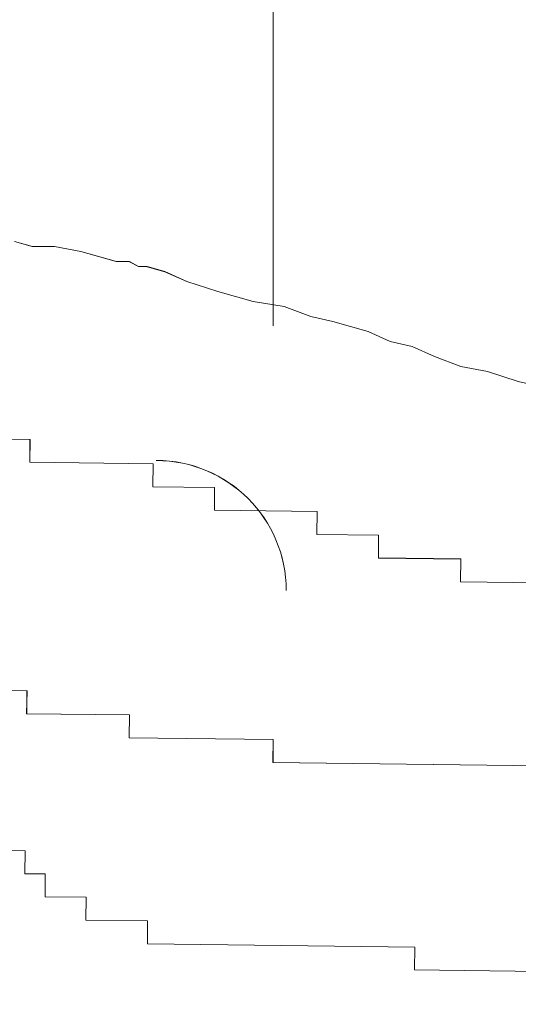
# Model space of a CAD drawing. Units: inches. Extents: x -466983 to 1020, y 324 to 318697.
# Tile 61 of 97: x 634.801 to 637.815, y 942.694 to 948.644. Entities that reach past the tile are written whole.
import ezdxf

# ---------------------------------------------------------------- set-up
doc = ezdxf.new("R2010")
doc.units = ezdxf.units.IN
doc.header["$MEASUREMENT"] = 0
doc.layers.add('A-FLOR-PATT', color=252, linetype='Continuous', lineweight=13)
doc.layers.add('A-FURN', color=8, linetype='Continuous', lineweight=18)

# ---------------------------------------------------------------- blocks, each defined once
blk = doc.blocks.new('L Shaped Sofa')
at = {"ltscale": 2}
for p, q in [((2423.757, 743.446), (2430.788, 743.36)), ((2430.788, 743.36), (2430.785, 743.108)), ((2430.785, 743.108), (2433.734, 743.072)), ((2433.734, 743.072), (2433.731, 742.82)), ((2433.731, 742.82), (2434.412, 742.812)), ((2434.412, 742.812), (2434.409, 742.56)), ((2434.409, 742.56), (2434.862, 742.555)), ((2434.862, 742.555), (2434.859, 742.303)), ((2434.859, 742.303), (2435.086, 742.3)), ((2435.086, 742.3), (2435.083, 742.048)), ((2435.083, 742.048), (2435.764, 742.04)), ((2421.46, 741.207), (2432.349, 741.074)), ((2432.349, 741.074), (2432.346, 740.822)), ((2432.346, 740.822), (2433.933, 740.802)), ((2433.933, 740.802), (2433.93, 740.55)), ((2433.93, 740.55), (2435.065, 740.536)), ((2435.065, 740.536), (2435.061, 740.285)), ((2435.061, 740.285), (2435.515, 740.279)), ((2428.468, 739.105), (2430.282, 739.083)), ((2430.282, 739.083), (2430.279, 738.831)), ((2430.279, 738.831), (2431.187, 738.82)), ((2431.187, 738.82), (2431.184, 738.568)), ((2431.184, 738.568), (2431.864, 738.56)), ((2431.864, 738.56), (2431.861, 738.308)), ((2431.861, 738.308), (2432.995, 738.294)), ((2432.995, 738.294), (2432.992, 738.042)), ((2432.992, 738.042), (2433.673, 738.034)), ((2433.673, 738.034), (2433.67, 737.782)), ((2433.67, 737.782), (2435.031, 737.765)), ((2435.031, 737.765), (2435.028, 737.514)), ((2435.028, 737.514), (2436.389, 737.497)), ((2429.4, 736.93), (2429.644, 736.875)), ((2429.644, 736.875), (2429.985, 736.765)), ((2429.985, 736.765), (2430.277, 736.709)), ((2430.277, 736.709), (2430.569, 736.599)), ((2430.569, 736.599), (2430.813, 736.49)), ((2430.813, 736.49), (2431.056, 736.434)), ((2431.056, 736.434), (2431.3, 736.325)), ((2431.3, 736.325), (2431.689, 736.215)), ((2431.689, 736.215), (2431.933, 736.159)), ((2432.347, 728.35), (2432.347, 736.259)), ((2431.933, 736.159), (2432.225, 736.049)), ((2432.225, 736.049), (2432.566, 735.994)), ((2432.566, 735.994), (2432.956, 735.883)), ((2432.956, 735.883), (2433.297, 735.773)), ((2433.297, 735.773), (2433.54, 735.664)), ((2433.54, 735.664), (2433.735, 735.609)), ((2433.735, 735.609), (2433.833, 735.608)), ((2433.833, 735.608), (2433.93, 735.554)), ((2433.93, 735.554), (2434.076, 735.553)), ((2434.076, 735.553), (2434.466, 735.443)), ((2434.466, 735.443), (2434.758, 735.387)), ((2434.758, 735.387), (2435.002, 735.386)), ((2435.002, 735.386), (2435.197, 735.331))]:
    blk.add_line(p, q, dxfattribs=at)
blk.add_arc((2433.636, 739.178), 1.433, 180, 270, dxfattribs=at)

msp = doc.modelspace()

# ---------------------------------------------------------------- hatches: boundary and pattern name
at = {"layer": 'A-FLOR-PATT', "transparency": 33554572}
h = msp.add_hatch(dxfattribs=at)
h.set_pattern_fill('ANSI37', color=256, scale=30)
h.set_pattern_definition([(45, (-1212.4137, -290.035), (-2.6516504, 2.6516504), []), (135, (-1212.4137, -290.035), (-2.6516504, -2.6516504), [])])
h.paths.add_polyline_path([(901.8057, 1075.9377), (900.6144, 1075.9377), (900.6144, 1065.3856), (899.391, 1065.3856), (898.0911, 1065.3856), (892.8356, 1058.7098, -0.258377), (892.1875, 1058.3509), (879.9848, 1058.3509, -0.20177), (879.4382, 1058.5808), (874.0812, 1065.3856), (872.7813, 1065.3856), (871.5579, 1065.3856), (871.5579, 1075.9377), (813.8057, 1075.9377), (813.8057, 1044.7922), (832.3947, 1044.7922, -0.394795), (848.6602, 1028.5356), (848.6602, 1009.9377), (901.8057, 1009.9377), (901.8057, 1015.9377), (901.3057, 1015.9377), (871.3057, 1015.9377), (871.3057, 1017.2502), (871.3344, 1017.2502, -0.401453), (901.3057, 1045.9377), (901.8057, 1045.9377)])
edge = h.paths.add_edge_path(flags=16)
edge.add_line((847.7731, 1068.9486), (847.7731, 1073.7088))
edge.add_arc((849.2269, 1073.7088), 1.4538, 90, 180, ccw=False)
edge.add_line((849.2269, 1075.1627), (864.4921, 1075.1627))
edge.add_arc((864.4921, 1073.7088), 1.4538, 0, 90, ccw=False)
edge.add_line((865.9459, 1073.7088), (865.9459, 1069.0035))
edge.add_arc((832.6447, 1068.9761), 33.3012, -20.61234, 0.04725, ccw=False)
edge.add_ellipse((856.8595, 1058.48), major_axis=(0, 10.2131), ratio=0.6859192, start_angle=100.00884, end_angle=259.99116, ccw=False)
edge.add_arc((881.0742, 1068.9761), 33.3012, 180.04725, 200.61234, ccw=False)
h.paths.add_polyline_path([(853.1456, 1066.4815), (853.1456, 1066.4534), (853.1463, 1066.4534, 0.433107), (852.9166, 1066.6849), (852.9166, 1066.4534), (853.1456, 1066.4534), (853.1456, 1066.4815), (853.088, 1066.6122, 0.697939), (852.6995, 1066.4534), (852.7003, 1066.4534), (852.7003, 1066.4815), (852.9166, 1067.0012), (852.9166, 1066.6849, -0.396254)], flags=0)
h.paths.add_polyline_path([(861.0187, 1066.4815), (861.0187, 1066.4534), (861.0194, 1066.4534, 0.416404), (860.8024, 1066.6849), (860.8024, 1066.4534), (861.0187, 1066.4534), (861.0187, 1066.4815), (860.9672, 1066.6053, 0.713344), (860.5726, 1066.4534), (860.5734, 1066.4534), (860.5734, 1066.4815), (860.8024, 1067.0012), (860.8024, 1066.6849, -0.379973)], flags=0)
edge = h.paths.add_edge_path(flags=0)
edge.add_spline(control_points=[(861.1298, 1065.7855), (861.4661, 1065.2478), (861.6134, 1065.0161), (861.9833, 1064.3736), (862.1924, 1063.9443), (862.5614, 1063.0391), (862.7212, 1062.5633), (862.9865, 1061.5781), (863.092, 1061.0689), (863.2452, 1060.031), (863.293, 1059.5025), (863.3295, 1058.4409), (863.3181, 1057.9078), (863.2366, 1056.8518), (863.1664, 1056.3289), (862.9695, 1055.308), (862.8427, 1054.8099), (862.5365, 1053.8522), (862.3571, 1053.3927), (861.9514, 1052.5249), (861.7251, 1052.1166), (861.233, 1051.3622), (860.9672, 1051.0162), (860.4048, 1050.3949), (860.1082, 1050.1197), (859.4937, 1049.6461), (859.1758, 1049.4476), (858.5276, 1049.1299), (858.1973, 1049.0107), (857.5315, 1048.8518), (857.1959, 1048.8121), (856.5249, 1048.812), (856.1894, 1048.8515), (855.5236, 1049.0101), (855.1933, 1049.1291), (854.545, 1049.4465), (854.2271, 1049.6449), (853.6124, 1050.1183), (853.3158, 1050.3933), (852.7533, 1051.0143), (852.4874, 1051.3602), (851.9952, 1052.1144), (851.7688, 1052.5225), (851.3629, 1053.3902), (851.1834, 1053.8496), (850.877, 1054.8071), (850.7501, 1055.3051), (850.553, 1056.326), (850.4827, 1056.8488), (850.401, 1057.9048), (850.3895, 1058.4379), (850.4257, 1059.4995), (850.4734, 1060.0281), (850.6265, 1061.066), (850.7318, 1061.5753), (850.9969, 1062.5605), (851.1567, 1063.0365), (851.5254, 1063.9418), (851.7345, 1064.3712), (852.1056, 1065.0164), (852.2544, 1065.2503), (852.6082, 1065.7335)], knot_values=[3.915332, 3.915332, 3.915332, 3.915332, 4.013468, 4.013468, 4.175532, 4.175532, 4.337596, 4.337596, 4.49966, 4.49966, 4.661724, 4.661724, 4.823788, 4.823788, 4.985852, 4.985852, 5.147916, 5.147916, 5.30998, 5.30998, 5.472044, 5.472044, 5.634109, 5.634109, 5.796173, 5.796173, 5.958237, 5.958237, 6.120301, 6.120301, 6.282365, 6.282365, 6.444429, 6.444429, 6.606493, 6.606493, 6.768557, 6.768557, 6.930621, 6.930621, 7.092685, 7.092685, 7.254749, 7.254749, 7.416813, 7.416813, 7.578878, 7.578878, 7.740942, 7.740942, 7.903006, 7.903006, 8.06507, 8.06507, 8.227134, 8.227134, 8.389198, 8.389198, 8.551262, 8.551262, 8.65037, 8.65037, 8.65037, 8.65037], degree=3, periodic=0)
edge.add_line((852.6421, 1065.7855), (861.1298, 1065.7855))
edge = h.paths.add_edge_path(flags=0)
edge.add_ellipse((856.8496, 1057.7432), major_axis=(0, 7.7921), ratio=0.687861, start_angle=0, end_angle=360)
h.paths.add_polyline_path([(848.8634, 1069.3891), (848.8634, 1073.9605, -0.414214), (849.9538, 1075.0508), (863.7652, 1075.0508, -0.414214), (864.8555, 1073.9605), (864.8555, 1069.3891, -0.388936), (864.5237, 1069.027, -0.043561), (849.1953, 1069.027, -0.388936)], flags=0)
h.paths.add_polyline_path([(853.1006, 1068.1122, -1), (852.6775, 1068.1122, -1)], flags=0)
edge = h.paths.add_edge_path(flags=0)
edge.add_ellipse((856.8595, 1057.3378), major_axis=(0, 2.207), ratio=0.657164, start_angle=0, end_angle=360)
h.paths.add_polyline_path([(861.0415, 1068.1122, -1), (860.6184, 1068.1122, -1)], flags=0)
edge = h.paths.add_edge_path()
edge.add_line((573.9537, 1057.3412), (573.9537, 1075.9377))
edge.add_line((573.9537, 1075.9377), (558.7308, 1075.9377))
edge.add_line((558.7308, 1075.9377), (558.7308, 1065.3856))
edge.add_line((558.7308, 1065.3856), (557.5074, 1065.3856))
edge.add_line((557.5074, 1065.3856), (556.2075, 1065.3856))
edge.add_line((556.2075, 1065.3856), (550.952, 1058.7098))
edge.add_arc((550.3039, 1059.1155), 0.7646, 270, 327.94832, ccw=False)
edge.add_line((550.3039, 1058.3509), (538.1012, 1058.3509))
edge.add_arc((538.1012, 1059.1155), 0.7646, 224.3704, 270, ccw=False)
edge.add_line((537.5546, 1058.5808), (532.1976, 1065.3856))
edge.add_line((532.1976, 1065.3856), (530.8977, 1065.3856))
edge.add_line((530.8977, 1065.3856), (529.6743, 1065.3856))
edge.add_line((529.6743, 1065.3856), (529.6743, 1075.9377))
edge.add_line((529.6743, 1075.9377), (520.8057, 1075.9377))
edge.add_line((520.8057, 1075.9377), (520.8057, 1045.9377))
edge.add_line((520.8057, 1045.9377), (521.3057, 1045.9377))
edge.add_arc((521.3057, 1015.9377), 30, 2.50749, 90, ccw=False)
edge.add_line((551.277, 1017.2502), (551.3057, 1017.2502))
edge.add_line((551.3057, 1017.2502), (551.3057, 1015.9377))
edge.add_line((551.3057, 1015.9377), (520.8057, 1015.9377))
edge.add_line((520.8057, 1015.9377), (520.8057, 1009.9377))
edge.add_line((520.8057, 1009.9377), (559.1913, 1010.4022))
edge.add_arc((559.1913, 1011.856), 1.4538, 180, 270, ccw=False)
edge.add_line((557.7375, 1011.856), (557.7375, 1016.5613))
edge.add_arc((591.0386, 1016.5888), 33.3012, 159.38766, 180.04725, ccw=False)
edge.add_ellipse((566.8239, 1027.0848), major_axis=(0, 10.2131), ratio=0.6859192, start_angle=280.00884, end_angle=439.99116, ccw=False)
edge.add_arc((542.6091, 1016.5888), 33.3012, 0.04725, 20.61234, ccw=False)
edge.add_line((575.9103, 1016.6162), (575.9103, 1011.856))
edge.add_arc((574.4565, 1011.856), 1.4538, -90, 0, ccw=False)
edge.add_line((574.4565, 1010.4022), (608.8057, 1009.9377))
edge.add_line((608.8057, 1009.9377), (608.8057, 1041.0857))
edge.add_line((608.8057, 1041.0857), (590.2179, 1041.0857))
edge.add_arc((590.775, 1057.9074), 16.8309, 181.92775, 268.10321, ccw=False)
edge = h.paths.add_edge_path()
edge.add_ellipse((494.2443, 583.6204), major_axis=(0, 10.2131), ratio=0.6859192, start_angle=280.00884, end_angle=439.99116, ccw=False)
edge.add_arc((470.0296, 573.1243), 33.3012, 0.04725, 20.61234, ccw=False)
edge.add_line((503.3307, 573.1518), (503.3307, 568.3916))
edge.add_arc((501.8769, 568.3916), 1.4538, -90, 0, ccw=False)
edge.add_line((501.8769, 566.9377), (539.8057, 566.9377))
edge.add_line((539.8057, 566.9377), (539.8057, 572.9377))
edge.add_line((539.8057, 572.9377), (539.3057, 572.9377))
edge.add_line((539.3057, 572.9377), (509.3057, 572.9377))
edge.add_line((509.3057, 572.9377), (509.3057, 574.2502))
edge.add_line((509.3057, 574.2502), (509.3344, 574.2502))
edge.add_arc((539.3057, 572.9377), 30, 90, 177.49251, ccw=False)
edge.add_line((539.3057, 602.9377), (539.8057, 602.9377))
edge.add_line((539.8057, 602.9377), (539.8057, 626.9377))
edge.add_line((539.8057, 626.9377), (531.7718, 626.9377))
edge.add_line((531.7718, 626.9377), (531.7718, 616.3856))
edge.add_line((531.7718, 616.3856), (530.5484, 616.3856))
edge.add_line((530.5484, 616.3856), (529.2485, 616.3856))
edge.add_line((529.2485, 616.3856), (523.7105, 609.3509))
edge.add_line((523.7105, 609.3509), (510.7766, 609.3509))
edge.add_line((510.7766, 609.3509), (505.2386, 616.3856))
edge.add_line((505.2386, 616.3856), (503.9387, 616.3856))
edge.add_line((503.9387, 616.3856), (502.7153, 616.3856))
edge.add_line((502.7153, 616.3856), (502.7153, 626.9377))
edge.add_line((502.7153, 626.9377), (481.6983, 626.9377))
edge.add_line((481.6983, 626.9377), (481.6983, 610.995))
edge.add_arc((467.2703, 611.4728), 14.4359, 271.92775, 358.10321, ccw=False)
edge.add_line((467.7559, 597.0451), (451.8057, 597.0451))
edge.add_line((451.8057, 597.0451), (451.8057, 584.4035))
edge.add_line((451.8057, 584.4035), (451.8057, 566.9377))
edge.add_line((451.8057, 566.9377), (486.6117, 566.9377))
edge.add_arc((486.6117, 568.3916), 1.4538, 180, 270, ccw=False)
edge.add_line((485.1579, 568.3916), (485.1579, 573.0969))
edge.add_arc((518.4591, 573.1243), 33.3012, 159.38766, 180.04725, ccw=False)
h.paths.add_polyline_path([(836.2609, 1020.7328), (879.8898, 1020.7328), (879.8898, 1039.3902), (836.2609, 1039.3902)], flags=25)
h.paths.add_polyline_path([(549.9851, 1036.7492), (593.614, 1036.7492), (593.614, 1055.4065), (549.9851, 1055.4065)], flags=24)
h.paths.add_polyline_path([(475.123, 595.5959), (518.752, 595.5959), (518.752, 614.2532), (475.123, 614.2532)], flags=24)
h = msp.add_hatch(dxfattribs=at)
h.set_pattern_fill('ANSI37', color=256, scale=20)
h.set_pattern_definition([(45, (-1212.4137, -290.035), (-1.767767, 1.767767), []), (135, (-1212.4137, -290.035), (-1.767767, -1.767767), [])])
h.paths.add_polyline_path([(809.8057, 870.9377), (809.8057, 888.1519), (806.9985, 888.1519), (802.6624, 888.1519), (789.3832, 888.1519), (786.2846, 888.1519, -0.414214), (785.4991, 888.9374), (785.4991, 900.1959), (785.4991, 908.4696, -0.414214), (786.8082, 909.7787, -0.414214), (785.4991, 911.0878), (785.4991, 929.1015, -0.414214), (786.8082, 930.4106, -0.414214), (785.4991, 931.7197), (785.4991, 931.9039, -0.414214), (784.19, 930.5948), (766.7223, 930.5948, -0.412359), (765.4132, 931.8956, -0.413741), (764.1145, 930.5782), (744.5781, 930.422, -0.416556), (743.7864, 931.2075), (743.7864, 933.5153), (742.2154, 933.5153), (742.2154, 952.024, -0.001344), (743.7864, 952.1998), (743.7864, 953.9377), (678.5915, 953.9377), (678.5915, 951.1305), (678.5915, 946.7945), (678.5915, 933.5153), (678.5915, 930.4166, -0.414214), (677.806, 929.6312), (666.5475, 929.6312), (658.2738, 929.6312, -0.414214), (656.9647, 930.9403, -0.414214), (655.6556, 929.6312), (637.6419, 929.6312, -0.414214), (636.3328, 930.9403, -0.414214), (635.0237, 929.6312), (634.8395, 929.6312, -0.414214), (636.1486, 928.322), (636.1486, 910.8544, -0.412359), (634.8478, 909.5452, -0.413741), (636.1653, 908.2466), (636.3214, 888.7102, -0.416556), (635.5359, 887.9184), (633.2281, 887.9184), (633.2281, 886.3475), (614.7194, 886.3475, -0.001344), (614.5436, 887.9184), (612.8057, 887.9184), (612.8057, 834.9377), (612.8057, 752.9377), (612.8057, 748.9377), (612.8057, 697.9377), (654.8057, 697.9377), (654.8057, 701.9377), (715.8057, 701.9377), (715.8057, 737.4353), (774.2918, 737.4353), (774.2918, 795.9377), (809.8057, 795.9377)])
h.paths.add_polyline_path([(679.2761, 849.5757, 0.102523), (682.1475, 849.2608, -0.080461), (694.5428, 849.7725, -0.283899), (694.4822, 849.0082, 0.136605), (694.4068, 848.8103, -0.030441), (694.5428, 846.8929), (694.5428, 842.6198), (694.5428, 838.3466, -0.028219), (694.4246, 836.5684), (694.425, 836.5684, 0.196187), (694.4456, 836.2708, -0.302897), (694.5428, 835.467, -0.080461), (682.1475, 835.9787, 0.102523), (679.2761, 835.6638, -0.58611), (678.6457, 836.0169), (678.6457, 849.2227, -0.58611)], flags=16)
h.paths.add_polyline_path([(679.5173, 848.6515, 0.699597), (679.476, 848.6342, 1.20716), (679.1935, 848.7422, 0.010621)], flags=0)
h.paths.add_polyline_path([(679.4923, 836.5608, -0.013798), (679.9178, 836.6594, -0.071703), (682.8533, 837.1434, -0.165743), (682.1665, 839.1006), (682.1665, 842.6094), (682.1665, 846.0603, -0.240616), (683.4733, 848.6767, -0.068263), (693.9295, 849.0082), (693.7875, 848.7083), (693.7875, 849.0228, 0.067332), (683.4733, 848.6767, 0.240616), (682.1665, 846.0603), (682.1665, 842.6094), (682.1665, 839.1006, 0.23459), (683.461, 836.5513, 0.068093), (693.7875, 836.1955), (693.7875, 836.5104), (693.9296, 836.2102, -0.077215), (682.2421, 836.7815, 0.086627), (679.5283, 836.5701, -0.628402), (679.5029, 836.5735), (679.5029, 836.6071, 0.910458)], flags=0)
h.paths.add_polyline_path([(679.476, 848.6364), (679.2069, 848.647), (679.2069, 836.5718, 0.913566), (679.3645, 836.5861), (679.476, 836.5824)], flags=0)
h.paths.add_polyline_path([(679.2761, 829.8604, 0.102523), (682.1475, 829.5455, -0.080461), (694.5428, 830.0572, -0.283899), (694.4822, 829.2929, 0.136605), (694.4068, 829.095, -0.030441), (694.5428, 827.1776), (694.5428, 822.9045), (694.5428, 818.6314, -0.028219), (694.4246, 816.8531), (694.425, 816.8532, 0.196187), (694.4456, 816.5555, -0.302897), (694.5428, 815.7517, -0.080461), (682.1475, 816.2635, 0.102523), (679.2761, 815.9485, -0.58611), (678.6457, 816.3016), (678.6457, 829.5074, -0.58611)], flags=16)
h.paths.add_polyline_path([(679.5173, 828.9362, 0.699597), (679.476, 828.9189, 1.20716), (679.1935, 829.0269, 0.010621)], flags=0)
h.paths.add_polyline_path([(679.4923, 816.8456, -0.013798), (679.9178, 816.9441, -0.071703), (682.8533, 817.4281, -0.165743), (682.1665, 819.3853), (682.1665, 822.8941), (682.1665, 826.345, -0.240616), (683.4733, 828.9614, -0.068263), (693.9295, 829.2929), (693.7875, 828.9931), (693.7875, 829.3076, 0.067332), (683.4733, 828.9614, 0.240616), (682.1665, 826.345), (682.1665, 822.8941), (682.1665, 819.3853, 0.23459), (683.461, 816.836, 0.068093), (693.7875, 816.4802), (693.7875, 816.7952), (693.9296, 816.4949, -0.077215), (682.2421, 817.0662, 0.086627), (679.5283, 816.8549, -0.628402), (679.5029, 816.8582), (679.5029, 816.8918, 0.910458)], flags=0)
h.paths.add_polyline_path([(679.476, 828.9211), (679.2069, 828.9317), (679.2069, 816.8565, 0.913566), (679.3645, 816.8708), (679.476, 816.8671)], flags=0)
h.paths.add_polyline_path([(679.2761, 810.1451, 0.102523), (682.1475, 809.8302, -0.080461), (694.5428, 810.342, -0.3023), (694.4466, 809.5394, 0.10023), (694.4058, 809.3878, -0.03057), (694.5428, 807.4623), (694.5428, 803.1892), (694.5428, 798.9161, -0.03057), (694.4058, 796.9906, 0.10023), (694.4466, 796.839, -0.3023), (694.5428, 796.0365, -0.080461), (682.1475, 796.5482, 0.102523), (679.2761, 796.2333, -0.58611), (678.6457, 796.5863), (678.6457, 809.7921, -0.58611)], flags=16)
h.paths.add_polyline_path([(679.5173, 809.2417, 0.699597), (679.476, 809.2244, 1.20716), (679.1935, 809.3324, 0.010621)], flags=0)
h.paths.add_polyline_path([(679.4923, 797.151, -0.013798), (679.9178, 797.2496, -0.071703), (682.8533, 797.7336, -0.165743), (682.1665, 799.6908), (682.1665, 803.1996), (682.1665, 806.6505, -0.239349), (683.461, 809.2577, -0.072465), (694.4468, 809.5405, 0.197932), (694.425, 809.2405), (693.7875, 809.2985), (693.7875, 809.6135, 0.068093), (683.461, 809.2577, 0.239349), (682.1665, 806.6505), (682.1665, 803.1996), (682.1665, 799.6908, 0.235854), (683.4733, 797.1323, 0.067332), (693.7875, 796.7861), (693.7875, 797.1006), (694.425, 797.1586, 0.197932), (694.4468, 796.8586, -0.080419), (682.1557, 797.3795, 0.083867), (679.5283, 797.1603, -0.628402), (679.5029, 797.1637), (679.5029, 797.1973, 0.910458)], flags=0)
h.paths.add_polyline_path([(679.2069, 809.2372), (679.2069, 797.162, 0.913566), (679.3645, 797.1763), (679.476, 797.1726), (679.476, 809.2266)], flags=0)
h.paths.add_polyline_path([(695.3643, 853.2989), (728.2231, 853.2989), (728.2231, 771.1519), (695.3643, 771.1519)], flags=16)
h.paths.add_polyline_path([(696.0215, 852.6417), (727.5659, 852.6417), (727.5659, 771.809), (696.0215, 771.809)], flags=0)
h.paths.add_polyline_path([(679.2761, 788.7869, 0.102523), (682.1475, 788.472, -0.080461), (694.5428, 788.9837, -0.3023), (694.4466, 788.1812, 0.10023), (694.4058, 788.0296, -0.03057), (694.5428, 786.1041), (694.5428, 781.831), (694.5428, 777.5578, -0.03057), (694.4058, 775.6323, 0.10023), (694.4466, 775.4808, -0.3023), (694.5428, 774.6782, -0.080461), (682.1475, 775.19, 0.102523), (679.2761, 774.875, -0.58611), (678.6457, 775.2281), (678.6457, 788.4339, -0.58611)], flags=16)
h.paths.add_polyline_path([(679.5173, 787.8834, 0.699597), (679.476, 787.8662, 1.20716), (679.1935, 787.9742, 0.010621)], flags=0)
h.paths.add_polyline_path([(679.4923, 775.7928, -0.013798), (679.9178, 775.8914, -0.071703), (682.8533, 776.3753, -0.165743), (682.1665, 778.3325), (682.1665, 781.8414), (682.1665, 785.2922, -0.239349), (683.461, 787.8995, -0.072465), (694.4468, 788.1823, 0.197932), (694.425, 787.8823), (693.7875, 787.9403), (693.7875, 788.2553, 0.068093), (683.461, 787.8995, 0.239349), (682.1665, 785.2922), (682.1665, 781.8414), (682.1665, 778.3325, 0.235854), (683.4733, 775.7741, 0.067332), (693.7875, 775.4279), (693.7875, 775.7424), (694.425, 775.8004, 0.197932), (694.4468, 775.5004, -0.080419), (682.1557, 776.0212, 0.083867), (679.5283, 775.8021, -0.628402), (679.5029, 775.8054), (679.5029, 775.8391, 0.910458)], flags=0)
h.paths.add_polyline_path([(679.2069, 787.8789), (679.2069, 775.8038, 0.913566), (679.3645, 775.818), (679.476, 775.8144), (679.476, 787.8684)], flags=0)
h.paths.add_polyline_path([(704.641, 854.1204, -0.080461), (705.1527, 866.5157, 0.102523), (704.8378, 869.3871, -0.58611), (705.1908, 870.0174), (718.3966, 870.0174, -0.58611), (718.7496, 869.3871, 0.102523), (718.4347, 866.5157, -0.080461), (718.9465, 854.1204, -0.3023), (718.1439, 854.2166, 0.10023), (717.9924, 854.2574, -0.03057), (716.0668, 854.1204), (711.7937, 854.1204), (707.5206, 854.1204, -0.03057), (705.5951, 854.2574, 0.10023), (705.4435, 854.2166, -0.3023)], flags=16)
h.paths.add_polyline_path([(717.8462, 869.1459, 0.699597), (717.8289, 869.1872, 1.20716), (717.9369, 869.4697, 0.010621)], flags=0)
h.paths.add_polyline_path([(705.4631, 854.2164, -0.080419), (705.984, 866.5074, 0.083867), (705.7648, 869.1349, -0.628402), (705.7682, 869.1603), (705.8018, 869.1603, 0.910458), (705.7555, 869.1709, -0.013798), (705.8541, 868.7454, -0.071703), (706.3381, 865.8099, -0.165743), (708.2953, 866.4967), (711.8041, 866.4967), (715.255, 866.4967, -0.239349), (717.8622, 865.2022, -0.072465), (718.145, 854.2164, 0.197932), (717.845, 854.2382), (717.903, 854.8757), (718.218, 854.8757, 0.068093), (717.8622, 865.2022, 0.239349), (715.255, 866.4967), (711.8041, 866.4967), (708.2953, 866.4967, 0.235854), (705.7368, 865.1898, 0.067332), (705.3906, 854.8757), (705.7051, 854.8757), (705.7631, 854.2382, 0.197932)], flags=16)
h.paths.add_polyline_path([(705.7665, 869.4563, 0.913566), (705.7808, 869.2987), (705.7771, 869.1872), (717.8311, 869.1872), (717.8417, 869.4563)], flags=0)
h.paths.add_polyline_path([(729.0446, 842.6198), (729.0446, 846.8929, -0.03057), (729.1817, 848.8184, 0.10023), (729.1408, 848.9699, -0.3023), (729.0446, 849.7725, -0.080461), (741.4399, 849.2608, 0.102523), (744.3113, 849.5757, -0.58611), (744.9417, 849.2227), (744.9417, 836.0169, -0.58611), (744.3113, 835.6638, 0.102523), (741.4399, 835.9787, -0.080461), (729.0446, 835.467, -0.3023), (729.1408, 836.2696, 0.10023), (729.1817, 836.4211, -0.03057), (729.0446, 838.3466)], flags=16)
h.paths.add_polyline_path([(744.1115, 836.5846, 1.20716), (744.3939, 836.4766, 0.010621), (744.0701, 836.5673, 0.699597)], flags=0)
h.paths.add_polyline_path([(729.1407, 836.2684, 0.197932), (729.1624, 836.5684), (729.7999, 836.5104), (729.7999, 836.1955, 0.068093), (740.1264, 836.5513, 0.239349), (741.4209, 839.1585), (741.4209, 842.6094), (741.4209, 846.1182, 0.235854), (740.1141, 848.6767, 0.067332), (729.7999, 849.0228), (729.7999, 848.7083), (729.1624, 848.6503, 0.197932), (729.1407, 848.9504, -0.080419), (741.4317, 848.4295, 0.083867), (744.0591, 848.6486, -0.628402), (744.0845, 848.6453), (744.0845, 848.6117, 0.910458), (744.0951, 848.6579, -0.013798), (743.6696, 848.5594, -0.071703), (740.7341, 848.0754, -0.165743), (741.4209, 846.1182), (741.4209, 842.6094), (741.4209, 839.1585, -0.239349), (740.1264, 836.5513, -0.072465)], flags=0)
h.paths.add_polyline_path([(729.0446, 830.0572, -0.080461), (741.4399, 829.5455, 0.102523), (744.3113, 829.8604, -0.58611), (744.9417, 829.5074), (744.9417, 816.3016, -0.58611), (744.3113, 815.9485, 0.102523), (741.4399, 816.2635, -0.080461), (729.0446, 815.7517, -0.3023), (729.1408, 816.5543, 0.10023), (729.1817, 816.7058, -0.03057), (729.0446, 818.6314), (729.0446, 822.9045), (729.0446, 827.1776, -0.03057), (729.1817, 829.1031, 0.10023), (729.1408, 829.2547, -0.3023)], flags=16)
h.paths.add_polyline_path([(744.1115, 816.8693, 1.20716), (744.3939, 816.7613, 0.010621), (744.0701, 816.852, 0.699597)], flags=0)
h.paths.add_polyline_path([(729.1407, 829.2351, -0.080419), (741.4317, 828.7142, 0.083867), (744.0591, 828.9334, -0.628402), (744.0845, 828.93), (744.0845, 828.8964, 0.910458), (744.0951, 828.9427, -0.013798), (743.6696, 828.8441, -0.071703), (740.7341, 828.3601, -0.165743), (741.4209, 826.4029), (741.4209, 822.8941), (741.4209, 819.4432, -0.239349), (740.1264, 816.836, -0.072465), (729.1407, 816.5531, 0.197932), (729.1624, 816.8532), (729.7999, 816.7952), (729.7999, 816.4802, 0.068093), (740.1264, 816.836, 0.239349), (741.4209, 819.4432), (741.4209, 822.8941), (741.4209, 826.4029, 0.235854), (740.1141, 828.9614, 0.067332), (729.7999, 829.3076), (729.7999, 828.9931), (729.1624, 828.9351, 0.197932)], flags=16)
h.paths.add_polyline_path([(729.0446, 810.342, -0.080461), (741.4399, 809.8302, 0.102523), (744.3113, 810.1451, -0.58611), (744.9417, 809.7921), (744.9417, 796.5863, -0.58611), (744.3113, 796.2333, 0.102523), (741.4399, 796.5482, -0.080461), (729.0446, 796.0365, -0.283899), (729.1052, 796.8007, 0.136605), (729.1806, 796.9987, -0.030441), (729.0446, 798.9161), (729.0446, 803.1892), (729.0446, 807.4623, -0.028219), (729.1628, 809.2406), (729.1624, 809.2405, 0.196187), (729.1418, 809.5382, -0.302897)], flags=16)
h.paths.add_polyline_path([(744.1115, 797.1748, 1.20716), (744.3939, 797.0668, 0.010621), (744.0701, 797.1575, 0.699597)], flags=0)
h.paths.add_polyline_path([(741.3453, 809.0275, 0.086627), (744.0591, 809.2388, -0.628402), (744.0845, 809.2355), (744.0845, 809.2019, 0.910458), (744.0951, 809.2481, -0.013798), (743.6696, 809.1496, -0.071703), (740.7341, 808.6656, -0.165743), (741.4209, 806.7084), (741.4209, 803.1996), (741.4209, 799.7487, -0.240616), (740.1141, 797.1323, -0.068263), (729.658, 796.8008), (729.7999, 797.1006), (729.7999, 796.7861, 0.067332), (740.1141, 797.1323, 0.240616), (741.4209, 799.7487), (741.4209, 803.1996), (741.4209, 806.7084, 0.23459), (740.1264, 809.2577, 0.068093), (729.7999, 809.6135), (729.7999, 809.2985), (729.6578, 809.5988, -0.077215)], flags=0)
h.paths.add_polyline_path([(704.641, 770.3304, -0.283899), (705.4053, 770.2697, 0.136605), (705.6032, 770.1944, -0.030441), (707.5206, 770.3304), (711.7937, 770.3304), (716.0668, 770.3304, -0.028219), (717.8451, 770.2122), (717.845, 770.2126, 0.196187), (718.1427, 770.2331, -0.302897), (718.9465, 770.3304, -0.080461), (718.4347, 757.9351, 0.102523), (718.7496, 755.0637, -0.58611), (718.3966, 754.4333), (705.1908, 754.4333, -0.58611), (704.8378, 755.0637, 0.102523), (705.1527, 757.9351, -0.080461)], flags=16)
h.paths.add_polyline_path([(705.762, 755.3048, 0.699597), (705.7793, 755.2635, 1.20716), (705.6713, 754.9811, 0.010621)], flags=0)
h.paths.add_polyline_path([(705.4053, 769.717), (705.7051, 769.5751), (705.3906, 769.5751, 0.067332), (705.7368, 759.2609, 0.240616), (708.3532, 757.954), (711.8041, 757.954), (715.3129, 757.954, 0.23459), (717.8622, 759.2485, 0.068093), (718.218, 769.5751), (717.903, 769.5751), (718.2033, 769.7172, -0.077215), (717.632, 758.0297, 0.086627), (717.8433, 755.3159, -0.628402), (717.84, 755.2904), (717.8064, 755.2904, 0.910458), (717.8526, 755.2799, -0.013798), (717.7541, 755.7053, -0.071703), (717.2701, 758.6409, -0.165743), (715.3129, 757.954), (711.8041, 757.954), (708.3532, 757.954, -0.240616), (705.7368, 759.2609, -0.068263)], flags=0)
h.paths.add_polyline_path([(729.0446, 788.9837, -0.080461), (741.4399, 788.472, 0.102523), (744.3113, 788.7869, -0.58611), (744.9417, 788.4339), (744.9417, 775.2281, -0.58611), (744.3113, 774.875, 0.102523), (741.4399, 775.19, -0.080461), (729.0446, 774.6782, -0.283899), (729.1052, 775.4425, 0.136605), (729.1806, 775.6405, -0.030441), (729.0446, 777.5578), (729.0446, 781.831), (729.0446, 786.1041, -0.028219), (729.1628, 787.8823), (729.1624, 787.8823, 0.196187), (729.1418, 788.1799, -0.302897)], flags=16)
h.paths.add_polyline_path([(744.1115, 775.8165, 1.20716), (744.3939, 775.7086, 0.010621), (744.0701, 775.7993, 0.699597)], flags=0)
h.paths.add_polyline_path([(741.3453, 787.6692, 0.086627), (744.0591, 787.8806, -0.628402), (744.0845, 787.8773), (744.0845, 787.8437, 0.910458), (744.0951, 787.8899, -0.013798), (743.6696, 787.7913, -0.071703), (740.7341, 787.3074, -0.165743), (741.4209, 785.3502), (741.4209, 781.8414), (741.4209, 778.3905, -0.240616), (740.1141, 775.7741, -0.068263), (729.658, 775.4425), (729.7999, 775.7424), (729.7999, 775.4279, 0.067332), (740.1141, 775.7741, 0.240616), (741.4209, 778.3905), (741.4209, 781.8414), (741.4209, 785.3502, 0.23459), (740.1264, 787.8995, 0.068093), (729.7999, 788.2553), (729.7999, 787.9403), (729.6578, 788.2405, -0.077215)], flags=0)
h.paths.add_polyline_path([(744.1115, 848.6364), (744.1115, 836.5824), (744.3805, 836.5718), (744.3805, 848.647, 0.913566), (744.2229, 848.6327)], flags=0)
h.paths.add_polyline_path([(744.2229, 828.9174), (744.1115, 828.9211), (744.1115, 816.8671), (744.3805, 816.8565), (744.3805, 828.9317, 0.913566)], flags=0)
h.paths.add_polyline_path([(717.8311, 755.2635), (705.7771, 755.2635), (705.7665, 754.9945), (717.8417, 754.9945, 0.913566), (717.8274, 755.1521)], flags=0)
h.paths.add_polyline_path([(744.2229, 809.2229), (744.1115, 809.2266), (744.1115, 797.1726), (744.3805, 797.162), (744.3805, 809.2372, 0.913566)], flags=0)
h.paths.add_polyline_path([(744.1115, 787.8684), (744.1115, 775.8144), (744.3805, 775.8038), (744.3805, 787.8789, 0.913566), (744.2229, 787.8647)], flags=0)
h.paths.add_polyline_path([(678.8774, 877.1228), (737.6127, 877.1228), (737.6127, 899.5116), (678.8774, 899.5116)], flags=24)

# ---------------------------------------------------------------- linework, layer by layer
at = {"layer": 'A-FURN', "ltscale": 2}
for p, q in [((636.3328, 951.1305), (636.3328, 946.7945)), ((636.3328, 951.1305), (636.3328, 946.7945)), ((636.3328, 951.1305), (636.3328, 946.7945)), ((636.3328, 951.1305), (636.3328, 946.7945)), ((636.3328, 951.1305), (636.3328, 946.7945)), ((636.3328, 951.1305), (636.3328, 946.7945)), ((634.8771, 947.2734), (634.7702, 947.3036)), ((634.8771, 947.2734), (634.7702, 947.3036)), ((634.8771, 947.2734), (634.7702, 947.3036)), ((634.8771, 947.2734), (634.7702, 947.3036)), ((634.8771, 947.2734), (634.7702, 947.3036)), ((634.8771, 947.2734), (634.7702, 947.3036)), ((635.0108, 947.2728), (634.8771, 947.2734)), ((635.0108, 947.2728), (634.8771, 947.2734)), ((635.0108, 947.2728), (634.8771, 947.2734)), ((635.0108, 947.2728), (634.8771, 947.2734)), ((635.0108, 947.2728), (634.8771, 947.2734)), ((635.0108, 947.2728), (634.8771, 947.2734)), ((635.1711, 947.2423), (635.0108, 947.2728)), ((635.1711, 947.2423), (635.0108, 947.2728)), ((635.1711, 947.2423), (635.0108, 947.2728)), ((635.1711, 947.2423), (635.0108, 947.2728)), ((635.1711, 947.2423), (635.0108, 947.2728)), ((635.1711, 947.2423), (635.0108, 947.2728)), ((635.3848, 947.1818), (635.1711, 947.2423)), ((635.3848, 947.1818), (635.1711, 947.2423)), ((635.3848, 947.1818), (635.1711, 947.2423)), ((635.3848, 947.1818), (635.1711, 947.2423)), ((635.3848, 947.1818), (635.1711, 947.2423)), ((635.3848, 947.1818), (635.1711, 947.2423)), ((635.465, 947.1815), (635.3848, 947.1818)), ((635.465, 947.1815), (635.3848, 947.1818)), ((635.465, 947.1815), (635.3848, 947.1818)), ((635.465, 947.1815), (635.3848, 947.1818)), ((635.465, 947.1815), (635.3848, 947.1818)), ((635.465, 947.1815), (635.3848, 947.1818)), ((635.5183, 947.1515), (635.465, 947.1815)), ((635.5183, 947.1515), (635.465, 947.1815)), ((635.5183, 947.1515), (635.465, 947.1815)), ((635.5183, 947.1515), (635.465, 947.1815)), ((635.5183, 947.1515), (635.465, 947.1815)), ((635.5183, 947.1515), (635.465, 947.1815)), ((635.5718, 947.1512), (635.5183, 947.1515)), ((635.5718, 947.1512), (635.5183, 947.1515)), ((635.5718, 947.1512), (635.5183, 947.1515)), ((635.5718, 947.1512), (635.5183, 947.1515)), ((635.5718, 947.1512), (635.5183, 947.1515)), ((635.5718, 947.1512), (635.5183, 947.1515)), ((635.6787, 947.121), (635.5718, 947.1512)), ((635.6787, 947.121), (635.5718, 947.1512)), ((635.6787, 947.121), (635.5718, 947.1512)), ((635.6787, 947.121), (635.5718, 947.1512)), ((635.6787, 947.121), (635.5718, 947.1512)), ((635.6787, 947.121), (635.5718, 947.1512)), ((635.812, 947.0609), (635.6787, 947.121)), ((635.812, 947.0609), (635.6787, 947.121)), ((635.812, 947.0609), (635.6787, 947.121)), ((635.812, 947.0609), (635.6787, 947.121)), ((635.812, 947.0609), (635.6787, 947.121)), ((635.812, 947.0609), (635.6787, 947.121)), ((635.9989, 947.0006), (635.812, 947.0609)), ((635.9989, 947.0006), (635.812, 947.0609)), ((635.9989, 947.0006), (635.812, 947.0609)), ((635.9989, 947.0006), (635.812, 947.0609)), ((635.9989, 947.0006), (635.812, 947.0609)), ((635.9989, 947.0006), (635.812, 947.0609)), ((636.2126, 946.9402), (635.9989, 947.0006)), ((636.2126, 946.9402), (635.9989, 947.0006)), ((636.2126, 946.9402), (635.9989, 947.0006)), ((636.2126, 946.9402), (635.9989, 947.0006)), ((636.2126, 946.9402), (635.9989, 947.0006)), ((636.2126, 946.9402), (635.9989, 947.0006)), ((636.3996, 946.9096), (636.2126, 946.9402)), ((636.3996, 946.9096), (636.2126, 946.9402)), ((636.3996, 946.9096), (636.2126, 946.9402)), ((636.3996, 946.9096), (636.2126, 946.9402)), ((636.3996, 946.9096), (636.2126, 946.9402)), ((636.3996, 946.9096), (636.2126, 946.9402)), ((636.5598, 946.8494), (636.3996, 946.9096)), ((636.5598, 946.8494), (636.3996, 946.9096)), ((636.5598, 946.8494), (636.3996, 946.9096)), ((636.5598, 946.8494), (636.3996, 946.9096)), ((636.5598, 946.8494), (636.3996, 946.9096)), ((636.5598, 946.8494), (636.3996, 946.9096)), ((636.6933, 946.819), (636.5598, 946.8494)), ((636.6933, 946.819), (636.5598, 946.8494)), ((636.6933, 946.819), (636.5598, 946.8494)), ((636.6933, 946.819), (636.5598, 946.8494)), ((636.6933, 946.819), (636.5598, 946.8494)), ((636.6933, 946.819), (636.5598, 946.8494)), ((636.907, 946.7586), (636.6933, 946.819)), ((636.907, 946.7586), (636.6933, 946.819)), ((636.907, 946.7586), (636.6933, 946.819)), ((636.907, 946.7586), (636.6933, 946.819)), ((636.907, 946.7586), (636.6933, 946.819)), ((636.907, 946.7586), (636.6933, 946.819)), ((637.0404, 946.6985), (636.907, 946.7586)), ((637.0404, 946.6985), (636.907, 946.7586)), ((637.0404, 946.6985), (636.907, 946.7586)), ((637.0404, 946.6985), (636.907, 946.7586)), ((637.0404, 946.6985), (636.907, 946.7586)), ((637.0404, 946.6985), (636.907, 946.7586)), ((637.1739, 946.6682), (637.0404, 946.6985)), ((637.1739, 946.6682), (637.0404, 946.6985)), ((637.1739, 946.6682), (637.0404, 946.6985)), ((637.1739, 946.6682), (637.0404, 946.6985)), ((637.1739, 946.6682), (637.0404, 946.6985)), ((637.1739, 946.6682), (637.0404, 946.6985)), ((637.3073, 946.6081), (637.1739, 946.6682)), ((637.3073, 946.6081), (637.1739, 946.6682)), ((637.3073, 946.6081), (637.1739, 946.6682)), ((637.3073, 946.6081), (637.1739, 946.6682)), ((637.3073, 946.6081), (637.1739, 946.6682)), ((637.3073, 946.6081), (637.1739, 946.6682)), ((637.4675, 946.5479), (637.3073, 946.6081)), ((637.4675, 946.5479), (637.3073, 946.6081)), ((637.4675, 946.5479), (637.3073, 946.6081)), ((637.4675, 946.5479), (637.3073, 946.6081)), ((637.4675, 946.5479), (637.3073, 946.6081)), ((637.4675, 946.5479), (637.3073, 946.6081)), ((637.6278, 946.5174), (637.4675, 946.5479)), ((637.6278, 946.5174), (637.4675, 946.5479)), ((637.6278, 946.5174), (637.4675, 946.5479)), ((637.6278, 946.5174), (637.4675, 946.5479)), ((637.6278, 946.5174), (637.4675, 946.5479)), ((637.6278, 946.5174), (637.4675, 946.5479)), ((637.8147, 946.4571), (637.6278, 946.5174)), ((637.8147, 946.4571), (637.6278, 946.5174)), ((637.8147, 946.4571), (637.6278, 946.5174)), ((637.8147, 946.4571), (637.6278, 946.5174)), ((637.8147, 946.4571), (637.6278, 946.5174)), ((637.8147, 946.4571), (637.6278, 946.5174)), ((634.8632, 946.1069), (634.1171, 946.1161)), ((634.8632, 946.1069), (634.1171, 946.1161)), ((634.8632, 946.1069), (634.1171, 946.1161)), ((634.8632, 946.1069), (634.1171, 946.1161)), ((634.8632, 946.1069), (634.1171, 946.1161)), ((634.8632, 946.1069), (634.1171, 946.1161)), ((634.8616, 945.9688), (634.8632, 946.1069)), ((634.8616, 945.9688), (634.8632, 946.1069)), ((634.8616, 945.9688), (634.8632, 946.1069)), ((634.8616, 945.9688), (634.8632, 946.1069)), ((634.8616, 945.9688), (634.8632, 946.1069)), ((634.8616, 945.9688), (634.8632, 946.1069)), ((635.6077, 945.9597), (634.8616, 945.9688)), ((635.6077, 945.9597), (634.8616, 945.9688)), ((635.6077, 945.9597), (634.8616, 945.9688)), ((635.6077, 945.9597), (634.8616, 945.9688)), ((635.6077, 945.9597), (634.8616, 945.9688)), ((635.6077, 945.9597), (634.8616, 945.9688)), ((635.606, 945.8216), (635.6077, 945.9597)), ((635.606, 945.8216), (635.6077, 945.9597)), ((635.606, 945.8216), (635.6077, 945.9597)), ((635.606, 945.8216), (635.6077, 945.9597)), ((635.606, 945.8216), (635.6077, 945.9597)), ((635.606, 945.8216), (635.6077, 945.9597)), ((635.9791, 945.8171), (635.606, 945.8216)), ((635.9791, 945.8171), (635.606, 945.8216)), ((635.9791, 945.8171), (635.606, 945.8216)), ((635.9791, 945.8171), (635.606, 945.8216)), ((635.9791, 945.8171), (635.606, 945.8216)), ((635.9791, 945.8171), (635.606, 945.8216)), ((635.9774, 945.679), (635.9791, 945.8171)), ((635.9774, 945.679), (635.9791, 945.8171)), ((635.9774, 945.679), (635.9791, 945.8171)), ((635.9774, 945.679), (635.9791, 945.8171)), ((635.9774, 945.679), (635.9791, 945.8171)), ((635.9774, 945.679), (635.9791, 945.8171)), ((636.5992, 945.6714), (635.9774, 945.679)), ((636.5992, 945.6714), (635.9774, 945.679)), ((636.5992, 945.6714), (635.9774, 945.679)), ((636.5992, 945.6714), (635.9774, 945.679)), ((636.5992, 945.6714), (635.9774, 945.679)), ((636.5992, 945.6714), (635.9774, 945.679)), ((636.5975, 945.5333), (636.5992, 945.6714)), ((636.5975, 945.5333), (636.5992, 945.6714)), ((636.5975, 945.5333), (636.5992, 945.6714)), ((636.5975, 945.5333), (636.5992, 945.6714)), ((636.5975, 945.5333), (636.5992, 945.6714)), ((636.5975, 945.5333), (636.5992, 945.6714)), ((636.9705, 945.5287), (636.5975, 945.5333)), ((636.9705, 945.5287), (636.5975, 945.5333)), ((636.9705, 945.5287), (636.5975, 945.5333)), ((636.9705, 945.5287), (636.5975, 945.5333)), ((636.9705, 945.5287), (636.5975, 945.5333)), ((636.9705, 945.5287), (636.5975, 945.5333)), ((636.9688, 945.3906), (636.9705, 945.5287)), ((636.9688, 945.3906), (636.9705, 945.5287)), ((636.9688, 945.3906), (636.9705, 945.5287)), ((636.9688, 945.3906), (636.9705, 945.5287)), ((636.9688, 945.3906), (636.9705, 945.5287)), ((636.9688, 945.3906), (636.9705, 945.5287)), ((637.4663, 945.3845), (636.9688, 945.3906)), ((637.4663, 945.3845), (636.9688, 945.3906)), ((637.4663, 945.3845), (636.9688, 945.3906)), ((637.4663, 945.3845), (636.9688, 945.3906)), ((637.4663, 945.3845), (636.9688, 945.3906)), ((637.4663, 945.3845), (636.9688, 945.3906)), ((637.4646, 945.2464), (637.4663, 945.3845)), ((637.4646, 945.2464), (637.4663, 945.3845)), ((637.4646, 945.2464), (637.4663, 945.3845)), ((637.4646, 945.2464), (637.4663, 945.3845)), ((637.4646, 945.2464), (637.4663, 945.3845)), ((637.4646, 945.2464), (637.4663, 945.3845)), ((638.4594, 945.2343), (637.4646, 945.2464)), ((638.4594, 945.2343), (637.4646, 945.2464)), ((638.4594, 945.2343), (637.4646, 945.2464)), ((638.4594, 945.2343), (637.4646, 945.2464)), ((638.4594, 945.2343), (637.4646, 945.2464)), ((638.4594, 945.2343), (637.4646, 945.2464)), ((634.8447, 944.5878), (634.596, 944.5909)), ((634.8447, 944.5878), (634.596, 944.5909)), ((634.8447, 944.5878), (634.596, 944.5909)), ((634.8447, 944.5878), (634.596, 944.5909)), ((634.8447, 944.5878), (634.596, 944.5909)), ((634.8447, 944.5878), (634.596, 944.5909)), ((634.843, 944.4497), (634.8447, 944.5878)), ((634.843, 944.4497), (634.8447, 944.5878)), ((634.843, 944.4497), (634.8447, 944.5878)), ((634.843, 944.4497), (634.8447, 944.5878)), ((634.843, 944.4497), (634.8447, 944.5878)), ((634.843, 944.4497), (634.8447, 944.5878)), ((635.4648, 944.4421), (634.843, 944.4497)), ((635.4648, 944.4421), (634.843, 944.4497)), ((635.4648, 944.4421), (634.843, 944.4497)), ((635.4648, 944.4421), (634.843, 944.4497)), ((635.4648, 944.4421), (634.843, 944.4497)), ((635.4648, 944.4421), (634.843, 944.4497)), ((635.4631, 944.304), (635.4648, 944.4421)), ((635.4631, 944.304), (635.4648, 944.4421)), ((635.4631, 944.304), (635.4648, 944.4421)), ((635.4631, 944.304), (635.4648, 944.4421)), ((635.4631, 944.304), (635.4648, 944.4421)), ((635.4631, 944.304), (635.4648, 944.4421)), ((636.3336, 944.2934), (635.4631, 944.304)), ((636.3336, 944.2934), (635.4631, 944.304)), ((636.3336, 944.2934), (635.4631, 944.304)), ((636.3336, 944.2934), (635.4631, 944.304)), ((636.3336, 944.2934), (635.4631, 944.304)), ((636.3336, 944.2934), (635.4631, 944.304)), ((636.3319, 944.1553), (636.3336, 944.2934)), ((636.3319, 944.1553), (636.3336, 944.2934)), ((636.3319, 944.1553), (636.3336, 944.2934)), ((636.3319, 944.1553), (636.3336, 944.2934)), ((636.3319, 944.1553), (636.3336, 944.2934)), ((636.3319, 944.1553), (636.3336, 944.2934)), ((642.3009, 944.0824), (636.3319, 944.1553)), ((642.3009, 944.0824), (636.3319, 944.1553)), ((642.3009, 944.0824), (636.3319, 944.1553)), ((642.3009, 944.0824), (636.3319, 944.1553)), ((642.3009, 944.0824), (636.3319, 944.1553)), ((642.3009, 944.0824), (636.3319, 944.1553)), ((634.8329, 943.6211), (634.4598, 943.6257)), ((634.8329, 943.6211), (634.4598, 943.6257)), ((634.8329, 943.6211), (634.4598, 943.6257)), ((634.8329, 943.6211), (634.4598, 943.6257)), ((634.8329, 943.6211), (634.4598, 943.6257)), ((634.8329, 943.6211), (634.4598, 943.6257)), ((634.8312, 943.483), (634.8329, 943.6211)), ((634.8312, 943.483), (634.8329, 943.6211)), ((634.8312, 943.483), (634.8329, 943.6211)), ((634.8312, 943.483), (634.8329, 943.6211)), ((634.8312, 943.483), (634.8329, 943.6211)), ((634.8312, 943.483), (634.8329, 943.6211)), ((634.9555, 943.4815), (634.8312, 943.483)), ((634.9555, 943.4815), (634.8312, 943.483)), ((634.9555, 943.4815), (634.8312, 943.483)), ((634.9555, 943.4815), (634.8312, 943.483)), ((634.9555, 943.4815), (634.8312, 943.483)), ((634.9555, 943.4815), (634.8312, 943.483)), ((634.9538, 943.3434), (634.9555, 943.4815)), ((634.9538, 943.3434), (634.9555, 943.4815)), ((634.9538, 943.3434), (634.9555, 943.4815)), ((634.9538, 943.3434), (634.9555, 943.4815)), ((634.9538, 943.3434), (634.9555, 943.4815)), ((634.9538, 943.3434), (634.9555, 943.4815)), ((635.2026, 943.3404), (634.9538, 943.3434)), ((635.2026, 943.3404), (634.9538, 943.3434)), ((635.2026, 943.3404), (634.9538, 943.3434)), ((635.2026, 943.3404), (634.9538, 943.3434)), ((635.2026, 943.3404), (634.9538, 943.3434)), ((635.2026, 943.3404), (634.9538, 943.3434)), ((635.2009, 943.2023), (635.2026, 943.3404)), ((635.2009, 943.2023), (635.2026, 943.3404)), ((635.2009, 943.2023), (635.2026, 943.3404)), ((635.2009, 943.2023), (635.2026, 943.3404)), ((635.2009, 943.2023), (635.2026, 943.3404)), ((635.2009, 943.2023), (635.2026, 943.3404)), ((635.5739, 943.1977), (635.2009, 943.2023)), ((635.5739, 943.1977), (635.2009, 943.2023)), ((635.5739, 943.1977), (635.2009, 943.2023)), ((635.5739, 943.1977), (635.2009, 943.2023)), ((635.5739, 943.1977), (635.2009, 943.2023)), ((635.5739, 943.1977), (635.2009, 943.2023)), ((635.5723, 943.0596), (635.5739, 943.1977)), ((635.5723, 943.0596), (635.5739, 943.1977)), ((635.5723, 943.0596), (635.5739, 943.1977)), ((635.5723, 943.0596), (635.5739, 943.1977)), ((635.5723, 943.0596), (635.5739, 943.1977)), ((635.5723, 943.0596), (635.5739, 943.1977)), ((637.1889, 943.0398), (635.5723, 943.0596)), ((637.1889, 943.0398), (635.5723, 943.0596)), ((637.1889, 943.0398), (635.5723, 943.0596)), ((637.1889, 943.0398), (635.5723, 943.0596)), ((637.1889, 943.0398), (635.5723, 943.0596)), ((637.1889, 943.0398), (635.5723, 943.0596)), ((637.1872, 942.9017), (637.1889, 943.0398)), ((637.1872, 942.9017), (637.1889, 943.0398)), ((637.1872, 942.9017), (637.1889, 943.0398)), ((637.1872, 942.9017), (637.1889, 943.0398)), ((637.1872, 942.9017), (637.1889, 943.0398)), ((637.1872, 942.9017), (637.1889, 943.0398)), ((641.0422, 942.8546), (637.1872, 942.9017)), ((641.0422, 942.8546), (637.1872, 942.9017)), ((641.0422, 942.8546), (637.1872, 942.9017)), ((641.0422, 942.8546), (637.1872, 942.9017)), ((641.0422, 942.8546), (637.1872, 942.9017)), ((641.0422, 942.8546), (637.1872, 942.9017))]:
    msp.add_line(p, q, dxfattribs=at)
msp.add_arc((635.6261, 945.1942), 0.7855, 0, 90, dxfattribs=at)
msp.add_arc((635.6261, 945.1942), 0.7855, 0, 90, dxfattribs=at)
msp.add_arc((635.6261, 945.1942), 0.7855, 0, 90, dxfattribs=at)
msp.add_arc((635.6261, 945.1942), 0.7855, 0, 90, dxfattribs=at)
msp.add_arc((635.6261, 945.1942), 0.7855, 0, 90, dxfattribs=at)
msp.add_arc((635.6261, 945.1942), 0.7855, 0, 90, dxfattribs=at)

# ---------------------------------------------------------------- block references
at = {"layer": 'A-FURN', "xscale": 0.5482153745360612, "yscale": 0.5482153745360612, "zscale": 0.5482153745360612, "rotation": 180}
msp.add_blockref('L Shaped Sofa', (1969.7828, 1350.4232), dxfattribs=at)

doc.saveas('drawing.dxf')
